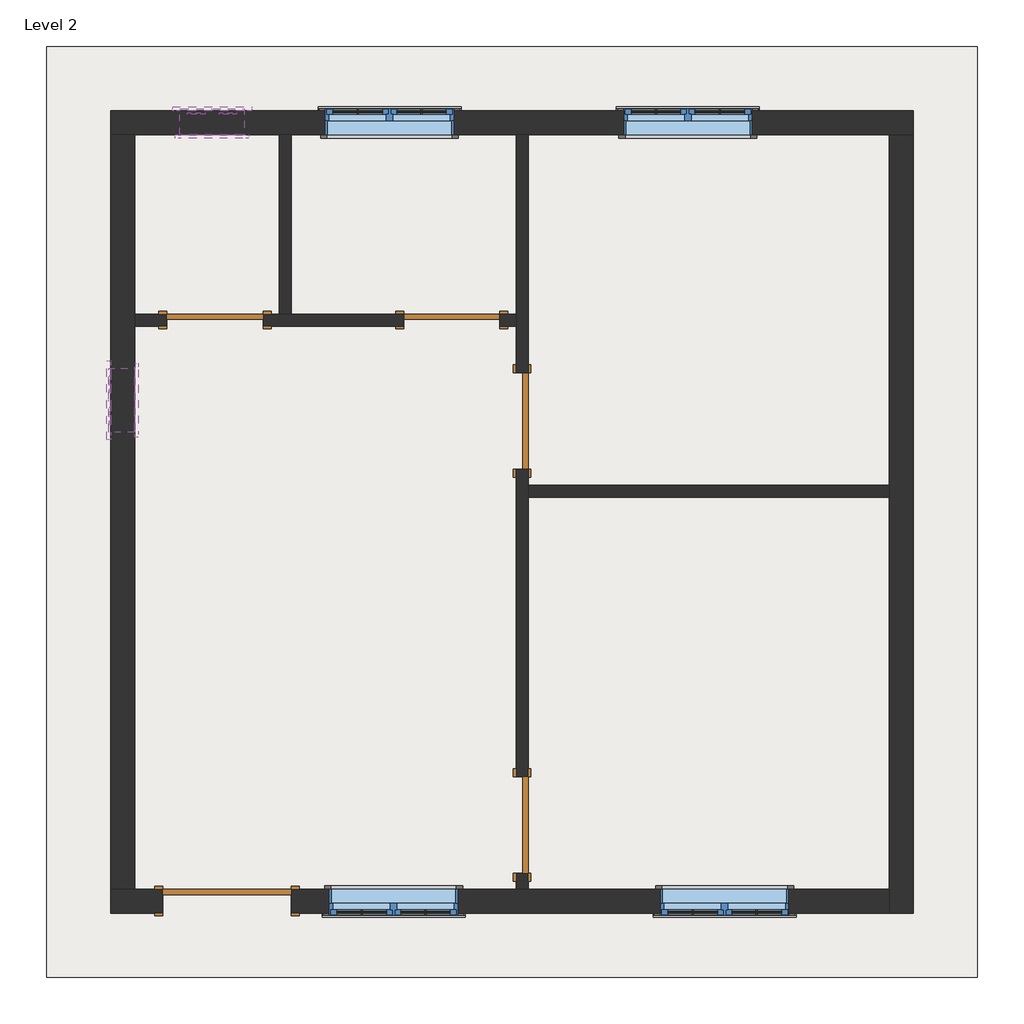
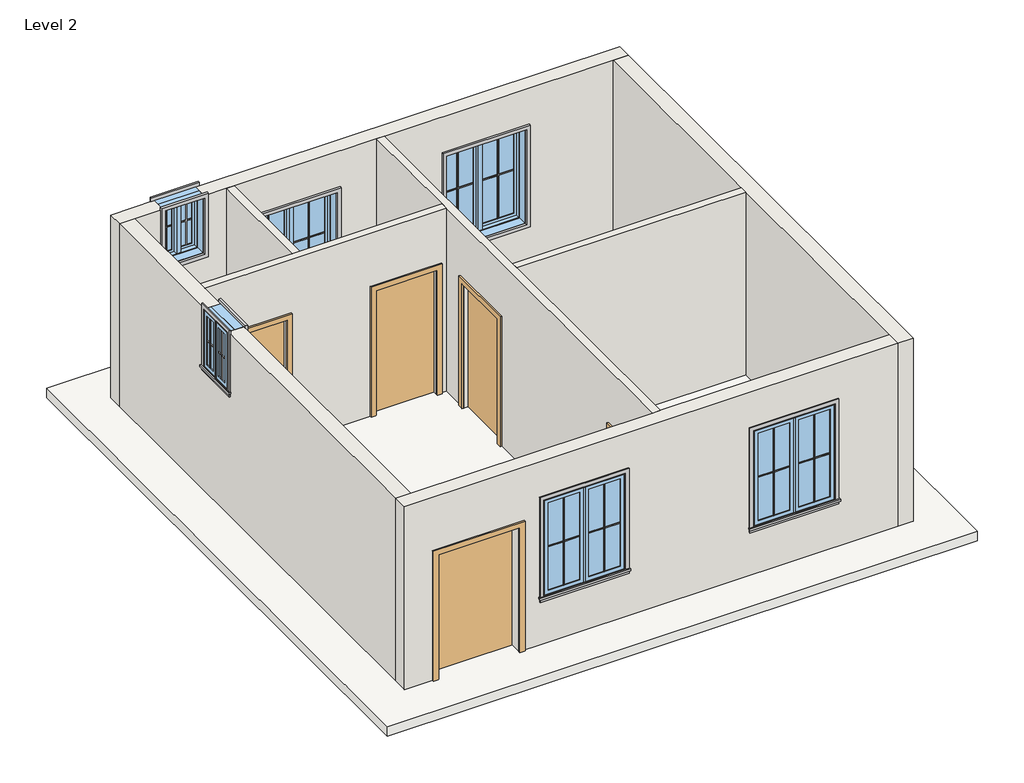
# One storey, incomplete: 24 proxies, 8 walls, 6 windows, 5 doors, 1 roof.
"""IFC4 building model written with IfcOpenShell, lengths in millimetres."""

from ifc_helpers import new_model, si_unit, frame, origin, place, context, project, spatial, polyline, outline, extrude, faceted_brep, transform, mapped, element, save
from components import muntin_pattern_2x2_muntin_pattern_2x2_6dad3731, muntin_pattern_2x2_muntin_pattern_2x2_a30a3345, muntin_pattern_2x2_muntin_pattern_2x2_53152e2c, muntin_pattern_2x2_muntin_pattern_2x2_e8f3e573, trim_window_exterior_flat_with_sill_92b9b949, trim_window_exterior_flat_with_sill_a665a915, trim_window_interior_flat_picture_frame_3bb882cf, trim_window_interior_flat_picture_frame_d485c387, door_e5f9f3c4, door_f4c4cdf2, window_c417fced, window_8377141f

model = new_model("IFC4")

# Units and contexts
model_context = context("Model", 3, world=origin())
ifc_project = project(units=[si_unit("LENGTHUNIT", "METRE", prefix="MILLI")], contexts=[model_context])

# Site, building, storey
site = spatial("IfcSite", under=ifc_project)
building = spatial("IfcBuilding", under=site)
storey = spatial("IfcBuildingStorey", under=building, Name="Level 2", Elevation=3048.0)

# Proxies
placement = place(None, origin())
muntin_pattern_2x2_muntin_pattern_2x2_shape = muntin_pattern_2x2_muntin_pattern_2x2_6dad3731(model_context)
element("IfcBuildingElementProxy", 1, Name="Muntin Pattern_2x2 : Muntin Pattern_2x2", ObjectType="Muntin Pattern_2x2 : Muntin Pattern_2x2", at=placement, inside=storey, context=model_context, shape_type="MappedRepresentation", body=[
    mapped(muntin_pattern_2x2_muntin_pattern_2x2_shape, transform((6192.8375, 13960.475, 4032.25), x_axis=(1.0, 0.0, 0.0), y_axis=(0.0, 1.0, 0.0), z_axis=(0.0, 0.0, 1.0))),
])
element("IfcBuildingElementProxy", 2, Name="Muntin Pattern_2x2 : Muntin Pattern_2x2", ObjectType="Muntin Pattern_2x2 : Muntin Pattern_2x2", at=placement, inside=storey, context=model_context, shape_type="MappedRepresentation", body=[
    mapped(muntin_pattern_2x2_muntin_pattern_2x2_shape, transform((7148.5125, 6359.525, 4032.25), x_axis=(-1.0, 0.0, 0.0), y_axis=(0.0, -1.0, 0.0), z_axis=(0.0, 0.0, 1.0))),
])
element("IfcBuildingElementProxy", 3, Name="Muntin Pattern_2x2 : Muntin Pattern_2x2", ObjectType="Muntin Pattern_2x2 : Muntin Pattern_2x2", at=placement, inside=storey, context=model_context, shape_type="MappedRepresentation", body=[
    mapped(muntin_pattern_2x2_muntin_pattern_2x2_shape, transform((4005.2625, 6359.525, 4032.25), x_axis=(-1.0, 0.0, 0.0), y_axis=(0.0, -1.0, 0.0), z_axis=(0.0, 0.0, 1.0))),
])
element("IfcBuildingElementProxy", 4, Name="Muntin Pattern_2x2 : Muntin Pattern_2x2", ObjectType="Muntin Pattern_2x2 : Muntin Pattern_2x2", at=placement, inside=storey, context=model_context, shape_type="MappedRepresentation", body=[
    mapped(muntin_pattern_2x2_muntin_pattern_2x2_shape, transform((3360.7375, 13960.475, 4032.25), x_axis=(1.0, 0.0, 0.0), y_axis=(0.0, 1.0, 0.0), z_axis=(0.0, 0.0, 1.0))),
])
muntin_pattern_2x2_muntin_pattern_2x2_2_shape = muntin_pattern_2x2_muntin_pattern_2x2_a30a3345(model_context)
element("IfcBuildingElementProxy", 5, Name="Muntin Pattern_2x2 : Muntin Pattern_2x2", ObjectType="Muntin Pattern_2x2 : Muntin Pattern_2x2", at=placement, inside=storey, context=model_context, shape_type="MappedRepresentation", body=[
    mapped(muntin_pattern_2x2_muntin_pattern_2x2_2_shape, transform((6799.2625, 13960.475, 4032.25), x_axis=(-1.0, 0.0, 0.0), y_axis=(0.0, -1.0, 0.0), z_axis=(0.0, 0.0, 1.0))),
])
element("IfcBuildingElementProxy", 6, Name="Muntin Pattern_2x2 : Muntin Pattern_2x2", ObjectType="Muntin Pattern_2x2 : Muntin Pattern_2x2", at=placement, inside=storey, context=model_context, shape_type="MappedRepresentation", body=[
    mapped(muntin_pattern_2x2_muntin_pattern_2x2_2_shape, transform((6542.0875, 6359.525, 4032.25), x_axis=(1.0, 0.0, 0.0), y_axis=(0.0, 1.0, 0.0), z_axis=(0.0, 0.0, 1.0))),
])
element("IfcBuildingElementProxy", 7, Name="Muntin Pattern_2x2 : Muntin Pattern_2x2", ObjectType="Muntin Pattern_2x2 : Muntin Pattern_2x2", at=placement, inside=storey, context=model_context, shape_type="MappedRepresentation", body=[
    mapped(muntin_pattern_2x2_muntin_pattern_2x2_2_shape, transform((3398.8375, 6359.525, 4032.25), x_axis=(1.0, 0.0, 0.0), y_axis=(0.0, 1.0, 0.0), z_axis=(0.0, 0.0, 1.0))),
])
element("IfcBuildingElementProxy", 8, Name="Muntin Pattern_2x2 : Muntin Pattern_2x2", ObjectType="Muntin Pattern_2x2 : Muntin Pattern_2x2", at=placement, inside=storey, context=model_context, shape_type="MappedRepresentation", body=[
    mapped(muntin_pattern_2x2_muntin_pattern_2x2_2_shape, transform((3967.1625, 13960.475, 4032.25), x_axis=(-1.0, 0.0, 0.0), y_axis=(0.0, -1.0, 0.0), z_axis=(0.0, 0.0, 1.0))),
])
muntin_pattern_2x2_muntin_pattern_2x2_3_shape = muntin_pattern_2x2_muntin_pattern_2x2_53152e2c(model_context)
element("IfcBuildingElementProxy", 9, Name="Muntin Pattern_2x2 : Muntin Pattern_2x2", ObjectType="Muntin Pattern_2x2 : Muntin Pattern_2x2", at=placement, inside=storey, context=model_context, shape_type="MappedRepresentation", body=[
    mapped(muntin_pattern_2x2_muntin_pattern_2x2_3_shape, transform((1025.525, 11069.6375, 5251.45), x_axis=(0.0, 1.0, 0.0), y_axis=(-1.0, 0.0, 0.0), z_axis=(0.0, 0.0, 1.0))),
])
element("IfcBuildingElementProxy", 10, Name="Muntin Pattern_2x2 : Muntin Pattern_2x2", ObjectType="Muntin Pattern_2x2 : Muntin Pattern_2x2", at=placement, inside=storey, context=model_context, shape_type="MappedRepresentation", body=[
    mapped(muntin_pattern_2x2_muntin_pattern_2x2_3_shape, transform((1827.2125, 13960.475, 5251.45), x_axis=(1.0, 0.0, 0.0), y_axis=(0.0, 1.0, 0.0), z_axis=(0.0, 0.0, 1.0))),
])
muntin_pattern_2x2_muntin_pattern_2x2_4_shape = muntin_pattern_2x2_muntin_pattern_2x2_e8f3e573(model_context)
element("IfcBuildingElementProxy", 11, Name="Muntin Pattern_2x2 : Muntin Pattern_2x2", ObjectType="Muntin Pattern_2x2 : Muntin Pattern_2x2", at=placement, inside=storey, context=model_context, shape_type="MappedRepresentation", body=[
    mapped(muntin_pattern_2x2_muntin_pattern_2x2_4_shape, transform((1025.525, 11371.2625, 5251.45), x_axis=(0.0, -1.0, 0.0), y_axis=(1.0, 0.0, 0.0), z_axis=(0.0, 0.0, 1.0))),
])
element("IfcBuildingElementProxy", 12, Name="Muntin Pattern_2x2 : Muntin Pattern_2x2", ObjectType="Muntin Pattern_2x2 : Muntin Pattern_2x2", at=placement, inside=storey, context=model_context, shape_type="MappedRepresentation", body=[
    mapped(muntin_pattern_2x2_muntin_pattern_2x2_4_shape, transform((2128.8375, 13960.475, 5251.45), x_axis=(-1.0, 0.0, 0.0), y_axis=(0.0, -1.0, 0.0), z_axis=(0.0, 0.0, 1.0))),
])
trim_window_exterior_flat_with_sill_shape = trim_window_exterior_flat_with_sill_92b9b949(model_context)
element("IfcBuildingElementProxy", 13, Name="Trim-Window-Exterior-Flat : with Sill", ObjectType="Trim-Window-Exterior-Flat : with Sill", at=placement, inside=storey, context=model_context, shape_type="MappedRepresentation", body=[
    mapped(trim_window_exterior_flat_with_sill_shape, transform((6496.05, 13970.0, 5486.4), x_axis=(-1.0, 0.0, 0.0), y_axis=(0.0, 0.0, 1.0), z_axis=(0.0, 1.0, 0.0))),
])
element("IfcBuildingElementProxy", 14, Name="Trim-Window-Exterior-Flat : with Sill", ObjectType="Trim-Window-Exterior-Flat : with Sill", at=placement, inside=storey, context=model_context, shape_type="MappedRepresentation", body=[
    mapped(trim_window_exterior_flat_with_sill_shape, transform((6845.3, 6350.0, 5486.4), x_axis=(1.0, 0.0, 0.0), y_axis=(0.0, 0.0, 1.0), z_axis=(0.0, -1.0, 0.0))),
])
element("IfcBuildingElementProxy", 15, Name="Trim-Window-Exterior-Flat : with Sill", ObjectType="Trim-Window-Exterior-Flat : with Sill", at=placement, inside=storey, context=model_context, shape_type="MappedRepresentation", body=[
    mapped(trim_window_exterior_flat_with_sill_shape, transform((3702.05, 6350.0, 5486.4), x_axis=(1.0, 0.0, 0.0), y_axis=(0.0, 0.0, 1.0), z_axis=(0.0, -1.0, 0.0))),
])
element("IfcBuildingElementProxy", 16, Name="Trim-Window-Exterior-Flat : with Sill", ObjectType="Trim-Window-Exterior-Flat : with Sill", at=placement, inside=storey, context=model_context, shape_type="MappedRepresentation", body=[
    mapped(trim_window_exterior_flat_with_sill_shape, transform((3663.95, 13970.0, 5486.4), x_axis=(-1.0, 0.0, 0.0), y_axis=(0.0, 0.0, 1.0), z_axis=(0.0, 1.0, 0.0))),
])
trim_window_exterior_flat_with_sill_2_shape = trim_window_exterior_flat_with_sill_a665a915(model_context)
element("IfcBuildingElementProxy", 17, Name="Trim-Window-Exterior-Flat : with Sill", ObjectType="Trim-Window-Exterior-Flat : with Sill", at=placement, inside=storey, context=model_context, shape_type="MappedRepresentation", body=[
    mapped(trim_window_exterior_flat_with_sill_2_shape, transform((1016.0, 11220.45, 6096.0), x_axis=(0.0, -1.0, 0.0), y_axis=(0.0, 0.0, 1.0), z_axis=(-1.0, 0.0, 0.0))),
])
element("IfcBuildingElementProxy", 18, Name="Trim-Window-Exterior-Flat : with Sill", ObjectType="Trim-Window-Exterior-Flat : with Sill", at=placement, inside=storey, context=model_context, shape_type="MappedRepresentation", body=[
    mapped(trim_window_exterior_flat_with_sill_2_shape, transform((1978.025, 13970.0, 6096.0), x_axis=(-1.0, 0.0, 0.0), y_axis=(0.0, 0.0, 1.0), z_axis=(0.0, 1.0, 0.0))),
])
trim_window_interior_flat_picture_frame_shape = trim_window_interior_flat_picture_frame_3bb882cf(model_context)
element("IfcBuildingElementProxy", 19, Name="Trim-Window-Interior-Flat : Picture Frame", ObjectType="Trim-Window-Interior-Flat : Picture Frame", at=placement, inside=storey, context=model_context, shape_type="MappedRepresentation", body=[
    mapped(trim_window_interior_flat_picture_frame_shape, transform((6496.05, 13741.4, 5486.4), x_axis=(1.0, 0.0, 0.0), y_axis=(0.0, 0.0, 1.0), z_axis=(0.0, -1.0, 0.0))),
])
element("IfcBuildingElementProxy", 20, Name="Trim-Window-Interior-Flat : Picture Frame", ObjectType="Trim-Window-Interior-Flat : Picture Frame", at=placement, inside=storey, context=model_context, shape_type="MappedRepresentation", body=[
    mapped(trim_window_interior_flat_picture_frame_shape, transform((6845.3, 6578.6, 5486.4), x_axis=(-1.0, 0.0, 0.0), y_axis=(0.0, 0.0, 1.0), z_axis=(0.0, 1.0, 0.0))),
])
element("IfcBuildingElementProxy", 21, Name="Trim-Window-Interior-Flat : Picture Frame", ObjectType="Trim-Window-Interior-Flat : Picture Frame", at=placement, inside=storey, context=model_context, shape_type="MappedRepresentation", body=[
    mapped(trim_window_interior_flat_picture_frame_shape, transform((3702.05, 6578.6, 5486.4), x_axis=(-1.0, 0.0, 0.0), y_axis=(0.0, 0.0, 1.0), z_axis=(0.0, 1.0, 0.0))),
])
element("IfcBuildingElementProxy", 22, Name="Trim-Window-Interior-Flat : Picture Frame", ObjectType="Trim-Window-Interior-Flat : Picture Frame", at=placement, inside=storey, context=model_context, shape_type="MappedRepresentation", body=[
    mapped(trim_window_interior_flat_picture_frame_shape, transform((3663.95, 13741.4, 5486.4), x_axis=(1.0, 0.0, 0.0), y_axis=(0.0, 0.0, 1.0), z_axis=(0.0, -1.0, 0.0))),
])
trim_window_interior_flat_picture_frame_2_shape = trim_window_interior_flat_picture_frame_d485c387(model_context)
element("IfcBuildingElementProxy", 23, Name="Trim-Window-Interior-Flat : Picture Frame", ObjectType="Trim-Window-Interior-Flat : Picture Frame", at=placement, inside=storey, context=model_context, shape_type="MappedRepresentation", body=[
    mapped(trim_window_interior_flat_picture_frame_2_shape, transform((1244.6, 11220.45, 6096.0), x_axis=(0.0, 1.0, 0.0), y_axis=(0.0, 0.0, 1.0), z_axis=(1.0, 0.0, 0.0))),
])
element("IfcBuildingElementProxy", 24, Name="Trim-Window-Interior-Flat : Picture Frame", ObjectType="Trim-Window-Interior-Flat : Picture Frame", at=placement, inside=storey, context=model_context, shape_type="MappedRepresentation", body=[
    mapped(trim_window_interior_flat_picture_frame_2_shape, transform((1978.025, 13741.4, 6096.0), x_axis=(1.0, 0.0, 0.0), y_axis=(0.0, 0.0, 1.0), z_axis=(0.0, -1.0, 0.0))),
])

# Doors
door_shape = door_e5f9f3c4(model_context)
element("IfcDoor", 25, ObjectType="Single-Flush : 36\" x 84\"", at=placement, inside=storey, context=model_context, shape_type="MappedRepresentation", body=[
    mapped(door_shape, transform((2006.6, 11982.45, 3048.0), x_axis=(1.0, 0.0, 0.0), y_axis=(0.0, 1.0, 0.0), z_axis=(0.0, 0.0, 1.0))),
])
element("IfcDoor", 26, ObjectType="Single-Flush : 36\" x 84\"", at=placement, inside=storey, context=model_context, shape_type="MappedRepresentation", body=[
    mapped(door_shape, transform((4254.5, 11982.45, 3048.0), x_axis=(1.0, 0.0, 0.0), y_axis=(0.0, 1.0, 0.0), z_axis=(0.0, 0.0, 1.0))),
])
element("IfcDoor", 27, ObjectType="Single-Flush : 36\" x 84\"", at=placement, inside=storey, context=model_context, shape_type="MappedRepresentation", body=[
    mapped(door_shape, transform((4921.25, 11023.6, 3048.0), x_axis=(0.0, -1.0, 0.0), y_axis=(1.0, 0.0, 0.0), z_axis=(0.0, 0.0, 1.0))),
])
element("IfcDoor", 28, ObjectType="Single-Flush : 36\" x 84\"", at=placement, inside=storey, context=model_context, shape_type="MappedRepresentation", body=[
    mapped(door_shape, transform((4921.25, 7188.2, 3048.0), x_axis=(0.0, -1.0, 0.0), y_axis=(1.0, 0.0, 0.0), z_axis=(0.0, 0.0, 1.0))),
])
door_2_shape = door_f4c4cdf2(model_context)
element("IfcDoor", 29, ObjectType="Single-Flush : 48\" x 84\"", at=placement, inside=storey, context=model_context, shape_type="MappedRepresentation", body=[
    mapped(door_2_shape, transform((2120.9, 6464.3, 3048.0), x_axis=(-1.0, 0.0, 0.0), y_axis=(0.0, -1.0, 0.0), z_axis=(0.0, 0.0, 1.0))),
])

# Roof
element("IfcRoof", 30, ObjectType="Generic - 12\"", at=placement, inside=storey, context=model_context, shape_type="SweptSolid", body=[
    extrude(outline(polyline([(406.4, 14579.6), (9245.6, 14579.6), (9245.6, 5740.4), (406.4, 5740.4), (406.4, 14579.6)])), frame((0.0, 0.0, 3048.0), z_axis=(0.0, 0.0, 1.0), x_axis=(1.0, 0.0, 0.0)), (0.0, 0.0, 1.0), 152.4),
])

# Walls
element("IfcWall", 31, ObjectType="Generic - 5\"", at=placement, inside=storey, context=model_context, shape_type="SweptSolid", body=[
    extrude(outline(polyline([(2616.2, 12039.6), (2616.2, 13741.4), (2730.5, 13741.4), (2730.5, 12039.6), (2616.2, 12039.6)])), frame((0.0, 0.0, 3048.0), z_axis=(0.0, 0.0, 1.0), x_axis=(1.0, 0.0, 0.0)), (0.0, 0.0, 1.0), 3048.0),
])
element("IfcWall", 32, ObjectType="Generic - 5\"", at=placement, inside=storey, context=model_context, shape_type="Brep", body=[
    faceted_brep([(4711.7, 11925.3, 5181.6), (4711.7, 11925.3, 3048.0), (4864.1, 11925.3, 3048.0), (4864.1, 11925.3, 6096.0), (1244.6, 11925.3, 6096.0), (1244.6, 11925.3, 3048.0), (1549.4, 11925.3, 3048.0), (1549.4, 11925.3, 5181.6), (2463.8, 11925.3, 5181.6), (2463.8, 11925.3, 3048.0), (3797.3, 11925.3, 3048.0), (3797.3, 11925.3, 5181.6), (4864.1, 12039.6, 3048.0), (4711.7, 12039.6, 3048.0), (4711.7, 12039.6, 5181.6), (3797.3, 12039.6, 5181.6), (3797.3, 12039.6, 3048.0), (2730.5, 12039.6, 3048.0), (2616.2, 12039.6, 3048.0), (2463.8, 12039.6, 3048.0), (2463.8, 12039.6, 5181.6), (1549.4, 12039.6, 5181.6), (1549.4, 12039.6, 3048.0), (1244.6, 12039.6, 3048.0), (1244.6, 12039.6, 6096.0), (2616.2, 12039.6, 6096.0), (2730.5, 12039.6, 6096.0), (4864.1, 12039.6, 6096.0)], [[[0, 1, 2, 3, 4, 5, 6, 7, 8, 9, 10, 11]], [[12, 13, 14, 15, 16, 17, 18, 19, 20, 21, 22, 23, 24, 25, 26, 27]], [[6, 5, 23, 22]], [[10, 9, 19, 18, 17, 16]], [[2, 1, 13, 12]], [[4, 3, 27, 26, 25, 24]], [[5, 4, 24, 23]], [[3, 2, 12, 27]], [[20, 19, 9, 8]], [[21, 20, 8, 7]], [[22, 21, 7, 6]], [[14, 13, 1, 0]], [[15, 14, 0, 11]], [[16, 15, 11, 10]]]),
])
element("IfcWall", 33, ObjectType="Generic - 5\"", at=placement, inside=storey, context=model_context, shape_type="Brep", body=[
    faceted_brep([(4864.1, 6731.0, 5181.6), (4864.1, 6731.0, 3048.0), (4864.1, 6578.6, 3048.0), (4864.1, 6578.6, 6096.0), (4864.1, 11925.3, 6096.0), (4864.1, 12039.6, 6096.0), (4864.1, 13741.4, 6096.0), (4864.1, 13741.4, 3048.0), (4864.1, 12039.6, 3048.0), (4864.1, 11925.3, 3048.0), (4864.1, 11480.8, 3048.0), (4864.1, 11480.8, 5181.6), (4864.1, 10566.4, 5181.6), (4864.1, 10566.4, 3048.0), (4864.1, 7645.4, 3048.0), (4864.1, 7645.4, 5181.6), (4978.4, 6578.6, 3048.0), (4978.4, 6731.0, 3048.0), (4978.4, 6731.0, 5181.6), (4978.4, 7645.4, 5181.6), (4978.4, 7645.4, 3048.0), (4978.4, 10299.7, 3048.0), (4978.4, 10414.0, 3048.0), (4978.4, 10566.4, 3048.0), (4978.4, 10566.4, 5181.6), (4978.4, 11480.8, 5181.6), (4978.4, 11480.8, 3048.0), (4978.4, 13741.4, 3048.0), (4978.4, 13741.4, 6096.0), (4978.4, 10414.0, 6096.0), (4978.4, 10299.7, 6096.0), (4978.4, 6578.6, 6096.0)], [[[0, 1, 2, 3, 4, 5, 6, 7, 8, 9, 10, 11, 12, 13, 14, 15]], [[16, 17, 18, 19, 20, 21, 22, 23, 24, 25, 26, 27, 28, 29, 30, 31]], [[10, 9, 8, 7, 27, 26]], [[14, 13, 23, 22, 21, 20]], [[2, 1, 17, 16]], [[6, 5, 4, 3, 31, 30, 29, 28]], [[7, 6, 28, 27]], [[3, 2, 16, 31]], [[24, 23, 13, 12]], [[25, 24, 12, 11]], [[26, 25, 11, 10]], [[18, 17, 1, 0]], [[19, 18, 0, 15]], [[20, 19, 15, 14]]]),
])
element("IfcWall", 34, ObjectType="Generic - 5\"", at=placement, inside=storey, context=model_context, shape_type="SweptSolid", body=[
    extrude(outline(polyline([(8407.4, 10299.7), (4978.4, 10299.7), (4978.4, 10414.0), (8407.4, 10414.0), (8407.4, 10299.7)])), frame((0.0, 0.0, 3048.0), z_axis=(0.0, 0.0, 1.0), x_axis=(1.0, 0.0, 0.0)), (0.0, 0.0, 1.0), 3048.0),
])
element("IfcWall", 35, ObjectType="Generic - 8\"", at=placement, inside=storey, context=model_context, shape_type="Brep", body=[
    faceted_brep([(1016.0, 13741.4, 3048.0), (1244.6, 13741.4, 3048.0), (2616.2, 13741.4, 3048.0), (2730.5, 13741.4, 3048.0), (4864.1, 13741.4, 3048.0), (4978.4, 13741.4, 3048.0), (8407.4, 13741.4, 3048.0), (8636.0, 13741.4, 3048.0), (8636.0, 13741.4, 6096.0), (8407.4, 13741.4, 6096.0), (4978.4, 13741.4, 6096.0), (4864.1, 13741.4, 6096.0), (2730.5, 13741.4, 6096.0), (2616.2, 13741.4, 6096.0), (2282.825, 13741.4, 6096.0), (2282.825, 13741.4, 5181.6), (1673.225, 13741.4, 5181.6), (1673.225, 13741.4, 6096.0), (1244.6, 13741.4, 6096.0), (1016.0, 13741.4, 6096.0), (7105.65, 13741.4, 5486.4), (7105.65, 13741.4, 3962.4), (5886.45, 13741.4, 3962.4), (5886.45, 13741.4, 5486.4), (4273.55, 13741.4, 5486.4), (4273.55, 13741.4, 3962.4), (3054.35, 13741.4, 3962.4), (3054.35, 13741.4, 5486.4), (8636.0, 13970.0, 3048.0), (1016.0, 13970.0, 3048.0), (1016.0, 13970.0, 6096.0), (1673.225, 13970.0, 6096.0), (1673.225, 13970.0, 5181.6), (2282.825, 13970.0, 5181.6), (2282.825, 13970.0, 6096.0), (8636.0, 13970.0, 6096.0), (7105.65, 13970.0, 3962.4), (7105.65, 13970.0, 5486.4), (5886.45, 13970.0, 5486.4), (5886.45, 13970.0, 3962.4), (4273.55, 13970.0, 3962.4), (4273.55, 13970.0, 5486.4), (3054.35, 13970.0, 5486.4), (3054.35, 13970.0, 3962.4)], [[[0, 1, 2, 3, 4, 5, 6, 7, 8, 9, 10, 11, 12, 13, 14, 15, 16, 17, 18, 19], [20, 21, 22, 23], [24, 25, 26, 27]], [[28, 29, 30, 31, 32, 33, 34, 35], [36, 37, 38, 39], [40, 41, 42, 43]], [[7, 6, 5, 4, 3, 2, 1, 0, 29, 28]], [[8, 35, 34, 14, 13, 12, 11, 10, 9]], [[30, 19, 18, 17, 31]], [[8, 7, 28, 35]], [[0, 19, 30, 29]], [[21, 20, 37, 36]], [[22, 21, 36, 39]], [[23, 22, 39, 38]], [[20, 23, 38, 37]], [[25, 24, 41, 40]], [[26, 25, 40, 43]], [[27, 26, 43, 42]], [[24, 27, 42, 41]], [[33, 15, 14, 34]], [[15, 33, 32, 16]], [[16, 32, 31, 17]]]),
])
element("IfcWall", 36, ObjectType="Generic - 8\"", at=placement, inside=storey, context=model_context, shape_type="Brep", body=[
    faceted_brep([(8407.4, 13741.4, 3048.0), (8407.4, 10414.0, 3048.0), (8407.4, 10299.7, 3048.0), (8407.4, 6578.6, 3048.0), (8407.4, 6350.0, 3048.0), (8407.4, 6350.0, 6096.0), (8407.4, 6578.6, 6096.0), (8407.4, 10299.7, 6096.0), (8407.4, 10414.0, 6096.0), (8407.4, 13741.4, 6096.0), (8636.0, 13741.4, 3048.0), (8636.0, 13741.4, 6096.0), (8636.0, 6350.0, 6096.0), (8636.0, 6350.0, 3048.0)], [[[0, 1, 2, 3, 4, 5, 6, 7, 8, 9]], [[10, 11, 12, 13]], [[4, 3, 2, 1, 0, 10, 13]], [[9, 8, 7, 6, 5, 12, 11]], [[0, 9, 11, 10]], [[5, 4, 13, 12]]]),
])
element("IfcWall", 37, ObjectType="Generic - 8\"", at=placement, inside=storey, context=model_context, shape_type="Brep", body=[
    faceted_brep([(1511.3, 6578.6, 5181.6), (1511.3, 6578.6, 3048.0), (1244.6, 6578.6, 3048.0), (1016.0, 6578.6, 3048.0), (1016.0, 6578.6, 6096.0), (1244.6, 6578.6, 6096.0), (4864.1, 6578.6, 6096.0), (4978.4, 6578.6, 6096.0), (8407.4, 6578.6, 6096.0), (8407.4, 6578.6, 3048.0), (4978.4, 6578.6, 3048.0), (4864.1, 6578.6, 3048.0), (2730.5, 6578.6, 3048.0), (2730.5, 6578.6, 5181.6), (6235.7, 6578.6, 5486.4), (6235.7, 6578.6, 3962.4), (7454.9, 6578.6, 3962.4), (7454.9, 6578.6, 5486.4), (3092.45, 6578.6, 5486.4), (3092.45, 6578.6, 3962.4), (4311.65, 6578.6, 3962.4), (4311.65, 6578.6, 5486.4), (1016.0, 6350.0, 3048.0), (1511.3, 6350.0, 3048.0), (1511.3, 6350.0, 5181.6), (2730.5, 6350.0, 5181.6), (2730.5, 6350.0, 3048.0), (8407.4, 6350.0, 3048.0), (8407.4, 6350.0, 6096.0), (1016.0, 6350.0, 6096.0), (6235.7, 6350.0, 5486.4), (7454.9, 6350.0, 5486.4), (7454.9, 6350.0, 3962.4), (6235.7, 6350.0, 3962.4), (3092.45, 6350.0, 5486.4), (4311.65, 6350.0, 5486.4), (4311.65, 6350.0, 3962.4), (3092.45, 6350.0, 3962.4)], [[[0, 1, 2, 3, 4, 5, 6, 7, 8, 9, 10, 11, 12, 13], [14, 15, 16, 17], [18, 19, 20, 21]], [[22, 23, 24, 25, 26, 27, 28, 29], [30, 31, 32, 33], [34, 35, 36, 37]], [[3, 2, 1, 23, 22]], [[12, 11, 10, 9, 27, 26]], [[8, 7, 6, 5, 4, 29, 28]], [[9, 8, 28, 27]], [[4, 3, 22, 29]], [[24, 23, 1, 0]], [[25, 24, 0, 13]], [[26, 25, 13, 12]], [[15, 14, 30, 33]], [[16, 15, 33, 32]], [[17, 16, 32, 31]], [[14, 17, 31, 30]], [[19, 18, 34, 37]], [[20, 19, 37, 36]], [[21, 20, 36, 35]], [[18, 21, 35, 34]]]),
])
element("IfcWall", 38, ObjectType="Generic - 8\"", at=placement, inside=storey, context=model_context, shape_type="Brep", body=[
    faceted_brep([(1244.6, 6578.6, 3048.0), (1244.6, 11925.3, 3048.0), (1244.6, 12039.6, 3048.0), (1244.6, 13741.4, 3048.0), (1244.6, 13741.4, 6096.0), (1244.6, 12039.6, 6096.0), (1244.6, 11925.3, 6096.0), (1244.6, 11525.25, 6096.0), (1244.6, 11525.25, 5181.6), (1244.6, 10915.65, 5181.6), (1244.6, 10915.65, 6096.0), (1244.6, 6578.6, 6096.0), (1016.0, 13741.4, 3048.0), (1016.0, 6578.6, 3048.0), (1016.0, 6578.6, 6096.0), (1016.0, 10915.65, 6096.0), (1016.0, 10915.65, 5181.6), (1016.0, 11525.25, 5181.6), (1016.0, 11525.25, 6096.0), (1016.0, 13741.4, 6096.0)], [[[0, 1, 2, 3, 4, 5, 6, 7, 8, 9, 10, 11]], [[12, 13, 14, 15, 16, 17, 18, 19]], [[3, 2, 1, 0, 13, 12]], [[14, 11, 10, 15]], [[4, 19, 18, 7, 6, 5]], [[4, 3, 12, 19]], [[0, 11, 14, 13]], [[17, 8, 7, 18]], [[8, 17, 16, 9]], [[9, 16, 15, 10]]]),
])

# Windows
window_shape = window_c417fced(model_context)
element("IfcWindow", 39, ObjectType="Window-Casement-Double : 24\" x 36\"", at=placement, inside=storey, context=model_context, shape_type="MappedRepresentation", body=[
    mapped(window_shape, transform((1130.3, 11220.45, 4267.2), x_axis=(0.0, 1.0, 0.0), y_axis=(-1.0, 0.0, 0.0), z_axis=(0.0, 0.0, 1.0))),
])
element("IfcWindow", 40, ObjectType="Window-Casement-Double : 24\" x 36\"", at=placement, inside=storey, context=model_context, shape_type="MappedRepresentation", body=[
    mapped(window_shape, transform((1978.025, 13855.7, 4267.2), x_axis=(1.0, 0.0, 0.0), y_axis=(0.0, 1.0, 0.0), z_axis=(0.0, 0.0, 1.0))),
])
window_2_shape = window_8377141f(model_context)
element("IfcWindow", 41, ObjectType="Window-Casement-Double : 48\" x 60\"", at=placement, inside=storey, context=model_context, shape_type="MappedRepresentation", body=[
    mapped(window_2_shape, transform((6496.05, 13855.7, 3048.0), x_axis=(1.0, 0.0, 0.0), y_axis=(0.0, 1.0, 0.0), z_axis=(0.0, 0.0, 1.0))),
])
element("IfcWindow", 42, ObjectType="Window-Casement-Double : 48\" x 60\"", at=placement, inside=storey, context=model_context, shape_type="MappedRepresentation", body=[
    mapped(window_2_shape, transform((6845.3, 6464.3, 3048.0), x_axis=(-1.0, 0.0, 0.0), y_axis=(0.0, -1.0, 0.0), z_axis=(0.0, 0.0, 1.0))),
])
element("IfcWindow", 43, ObjectType="Window-Casement-Double : 48\" x 60\"", at=placement, inside=storey, context=model_context, shape_type="MappedRepresentation", body=[
    mapped(window_2_shape, transform((3702.05, 6464.3, 3048.0), x_axis=(-1.0, 0.0, 0.0), y_axis=(0.0, -1.0, 0.0), z_axis=(0.0, 0.0, 1.0))),
])
element("IfcWindow", 44, ObjectType="Window-Casement-Double : 48\" x 60\"", at=placement, inside=storey, context=model_context, shape_type="MappedRepresentation", body=[
    mapped(window_2_shape, transform((3663.95, 13855.7, 3048.0), x_axis=(1.0, 0.0, 0.0), y_axis=(0.0, 1.0, 0.0), z_axis=(0.0, 0.0, 1.0))),
])

save(model, "model.ifc")

# Revit data of these elements
# Type "Muntin Pattern_2x2 : Muntin Pattern_2x2"
#   Width [instance default] = 4' - 0"
#   Thickness = 0' - 0 1/2"
#   Height [instance default] = 4' - 0"
#   Distance = 0' - 0 3/4"
#   Interior Material [instance default] = none
#   Exterior Material [instance default] = none
#   Default Elevation = 0
# Type "Trim-Window-Exterior-Flat : with Sill"
#   Trim Width = 0' - 2 1/4"
#   Trim Thickness_Picture Frame = 0' - 1 1/4"
#   Trim Thickness_with Sill = 0' - 0 3/4"
#   Sill Thickness = 0' - 1 1/4"
#   Opening Width [instance default] = 2' - 0"
#   Opening Height [instance default] = 3' - 0"
#   Default Elevation = 4' - 0"
#   Sill = yes
#   Picture Frame = no
#   Trim Material [instance default] = none
# Type "Trim-Window-Interior-Flat : Picture Frame"
#   Trim Thickness_Picture Frame = 0' - 1 1/4"
#   Trim Width = 0' - 2 1/4"
#   Trim Thickness_with Sill = 0' - 0 3/4"
#   Sill Thickness = 0' - 1 1/4"
#   Opening Width [instance default] = 2' - 0"
#   Opening Height [instance default] = 3' - 0"
#   Default Elevation = 4' - 0"
#   Sill = no
#   Picture Frame = yes
#   Trim Material [instance default] = none
# Type "Single-Flush : 36\" x 84\""
#   Type Mark = "1"
#   Construction Type Id = "MDOOR"
#   Assembly Code = "C1020"
#   Analytic Construction = "Metal"
#   Thickness = 0' - 2"
#   Heat Transfer Coefficient (U) = 0.651978 BTU/(h·ft²·°F)
#   Height = 7' - 0"
#   Trim Projection Ext = 0' - 1"
#   Trim Projection Int = 0' - 1"
#   Trim Width = 0' - 3"
#   Width = 3' - 0"
#   Define Thermal Properties by = 1
#   Define Thermal Properties by = 1
#   Door Material = Door - Panel
#   Frame Material = Door - Frame
#   Visual Light Transmittance = 0
#   Solar Heat Gain Coefficient = 0
#   Function = (empty or 0)
#   Wall Closure = (empty or 0)
# Type "Single-Flush : 48\" x 84\""
#   Type Mark = "5"
#   Construction Type Id = "MDOOR"
#   Assembly Code = "C1020"
#   Analytic Construction = "Metal"
#   Thickness = 0' - 2"
#   Heat Transfer Coefficient (U) = 0.651978 BTU/(h·ft²·°F)
#   Height = 7' - 0"
#   Trim Projection Ext = 0' - 1"
#   Trim Projection Int = 0' - 1"
#   Trim Width = 0' - 3"
#   Width = 4' - 0"
#   Define Thermal Properties by = 1
#   Define Thermal Properties by = 1
#   Door Material = Door - Panel
#   Frame Material = Door - Frame
#   Visual Light Transmittance = 0
#   Solar Heat Gain Coefficient = 0
#   Function = (empty or 0)
#   Wall Closure = (empty or 0)
# Type "Generic - 12\""
#   Assembly Code = "B1020"
#   Layers, outside or top first: 0' - 6" no material (function 1)
# Type "Generic - 5\""
#   Assembly Code = "B2010"
#   Layers, outside or top first: 0' - 4 1/2" no material (function 1)
# Type "Generic - 8\""
#   Assembly Code = "B2010"
#   Layers, outside or top first: 0' - 9" "Parking Stripe" (function 1)
# Type "Window-Casement-Double : 24\" x 36\""
#   Type Mark = "14"
#   Fire Rating = "0.5h"
#   Assembly Code = "B2020100"
#   Analytic Construction = "Double glazing - domestic"
#   Frame Extension [instance default] = 0' - 0 1/4"
#   Window Inset [instance default] = 0' - 0"
#   Wall Thickness [instance default] = 0' - 6"
#   Interior Wall Closure [instance default] = 0' - 2 1/4"
#   Half Width = 1' - 0"
#   Visual Light Transmittance = 0.81
#   Thermal Resistance (R) = 1.8146 (h·ft²·°F)/BTU
#   Solar Heat Gain Coefficient = 0.76
#   Rough Width = 2' - 0 1/2"
#   Rough Height = 3' - 0 1/2"
#   Height = 3' - 0"
#   Heat Transfer Coefficient (U) = 0.5511 BTU/(h·ft²·°F)
#   Exterior Wall Closure [instance default] = 0' - 1 1/4"
#   Extension Jamb [instance default] = 0' - 2 1/4"
#   Default Sill Height = 3' - 0"
#   Width = 2' - 0"
#   Define Thermal Properties by = 0
#   Muntin Visibility = yes
#   Interior Trim Visibility [instance default] = yes
#   Exterior Trim Visibility [instance default] = yes
#   Extension Jamb Visibility [instance default] = yes
#   Interior Trim Material = Wood - Stained
#   Muntin Pattern = Muntin Pattern_2x2 : Muntin Pattern_2x2
#   Interior Trim = Trim-Window-Interior-Flat : Picture Frame
#   Interior Frame Material = Wood - Stained
#   Glass Panel Material = Glass
#   Exterior Trim Material = Clad - White
#   Exterior Trim = Trim-Window-Exterior-Flat : with Sill
#   Exterior Frame Material = Clad - White
#   Wall Closure = (empty or 0)
# Type "Window-Casement-Double : 48\" x 60\""
#   Type Mark = "17"
#   Fire Rating = "0.5h"
#   Assembly Code = "B2020100"
#   Analytic Construction = "Double glazing - domestic"
#   Frame Extension [instance default] = 0' - 0 1/4"
#   Window Inset [instance default] = 0' - 0"
#   Wall Thickness [instance default] = 0' - 6"
#   Interior Wall Closure [instance default] = 0' - 2 1/4"
#   Half Width = 2' - 0"
#   Visual Light Transmittance = 0.81
#   Thermal Resistance (R) = 1.8146 (h·ft²·°F)/BTU
#   Solar Heat Gain Coefficient = 0.76
#   Rough Width = 4' - 0 1/2"
#   Rough Height = 5' - 0 1/2"
#   Height = 5' - 0"
#   Heat Transfer Coefficient (U) = 0.5511 BTU/(h·ft²·°F)
#   Exterior Wall Closure [instance default] = 0' - 1 1/4"
#   Extension Jamb [instance default] = 0' - 2 1/4"
#   Default Sill Height = 3' - 0"
#   Width = 4' - 0"
#   Define Thermal Properties by = 0
#   Muntin Visibility = yes
#   Interior Trim Visibility [instance default] = yes
#   Exterior Trim Visibility [instance default] = yes
#   Extension Jamb Visibility [instance default] = yes
#   Interior Trim Material = Wood - Stained
#   Muntin Pattern = Muntin Pattern_2x2 : Muntin Pattern_2x2
#   Interior Trim = Trim-Window-Interior-Flat : Picture Frame
#   Interior Frame Material = Wood - Stained
#   Glass Panel Material = Glass
#   Exterior Trim Material = Clad - White
#   Exterior Trim = Trim-Window-Exterior-Flat : with Sill
#   Exterior Frame Material = Clad - White
#   Wall Closure = (empty or 0)
# Elements 1, 2, 3, 4, 5, 6, 7, 8 (IfcBuildingElementProxy, "Muntin Pattern_2x2 : Muntin Pattern_2x2")
#   Width = 1' - 6 5/8"
#   Height = 4' - 6 1/2"
#   Interior Material = Wood - Stained
#   Exterior Material = Clad - White
#   Phase Created = New Construction
#   Materials on its faces: "Clad - White", "Wood - Stained"
# Elements 9, 10, 11, 12 (IfcBuildingElementProxy, "Muntin Pattern_2x2 : Muntin Pattern_2x2")
#   Width = 0' - 6 5/8"
#   Height = 2' - 6 1/2"
#   Interior Material = Wood - Stained
#   Exterior Material = Clad - White
#   Phase Created = New Construction
#   Materials on its faces: "Clad - White", "Wood - Stained"
# Elements 13, 14, 15, 16 (IfcBuildingElementProxy, "Trim-Window-Exterior-Flat : with Sill")
#   Opening Width = 4' - 0"
#   Opening Height = 5' - 0"
#   Trim Material = Clad - White
#   Phase Created = New Construction
#   Materials on its faces: "Clad - White"
# Elements 17, 18 (IfcBuildingElementProxy, "Trim-Window-Exterior-Flat : with Sill")
#   Opening Width = 2' - 0"
#   Opening Height = 3' - 0"
#   Trim Material = Clad - White
#   Phase Created = New Construction
#   Materials on its faces: "Clad - White"
# Elements 19, 20, 21, 22 (IfcBuildingElementProxy, "Trim-Window-Interior-Flat : Picture Frame")
#   Opening Width = 4' - 0"
#   Opening Height = 5' - 0"
#   Trim Material = Wood - Stained
#   Phase Created = New Construction
#   Materials on its faces: "Wood - Stained"
# Elements 23, 24 (IfcBuildingElementProxy, "Trim-Window-Interior-Flat : Picture Frame")
#   Opening Width = 2' - 0"
#   Opening Height = 3' - 0"
#   Trim Material = Wood - Stained
#   Phase Created = New Construction
#   Materials on its faces: "Wood - Stained"
# Elements 25, 26, 27, 28 (IfcDoor, "Single-Flush : 36\" x 84\"")
#   Phase Created = New Construction
#   Materials on its faces: "Door - Frame", "Door - Panel"
# Element 29 (IfcDoor, "Single-Flush : 48\" x 84\"")
#   Phase Created = New Construction
#   Materials on its faces: "Door - Frame", "Door - Panel"
# Element 30 (IfcRoof, "Generic - 12\"")
#   built-in parameter 1001705 = 10.5 (stored number, unit not read)
#   built-in parameter 1001710 = 33615
#   Phase Created = New Construction
#   Materials on its faces: "Textile - Linen, Smooth", "Wood Planks"
# Elements 31, 32, 33, 34 (IfcWall, "Generic - 5\"")
#   Top Offset = 0' - 0"
#   Base Offset = 0' - 0"
#   wall height = 10' - 0"
#   Phase Created = New Construction
#   Base Constraint = Level 2
#   Top Constraint = Level 3
#   Materials on its faces: "Default Wall"
# Elements 35, 36, 37, 38 (IfcWall, "Generic - 8\"")
#   Top Offset = 0' - 0"
#   Base Offset = 0' - 0"
#   Unconnected Height = 10' - 0"
#   wall height = 10' - 0"
#   Phase Created = New Construction
#   Base Constraint = Level 2
#   Materials on its faces: "Parking Stripe", "Wood Planks"
# Element 39 (IfcWindow, "Window-Casement-Double : 24\" x 36\"")
#   Mark = "11"
#   Window Inset = 0' - 0"
#   Interior Wall Closure = 0' - 2 1/4"
#   Frame Extension = 0' - 0 1/4"
#   Exterior Wall Closure = 0' - 1 1/4"
#   Interior Trim Visibility = yes
#   Exterior Trim Visibility = yes
#   Phase Created = New Construction
#   Materials on its faces: "Wood - Stained", "Glass", "Clad - White"
# Element 40 (IfcWindow, "Window-Casement-Double : 24\" x 36\"")
#   Mark = "12"
#   Window Inset = 0' - 0"
#   Interior Wall Closure = 0' - 2 1/4"
#   Frame Extension = 0' - 0 1/4"
#   Exterior Wall Closure = 0' - 1 1/4"
#   Interior Trim Visibility = yes
#   Exterior Trim Visibility = yes
#   Phase Created = New Construction
#   Materials on its faces: "Wood - Stained", "Glass", "Clad - White"
# Element 41 (IfcWindow, "Window-Casement-Double : 48\" x 60\"")
#   Mark = "7"
#   Window Inset = 0' - 0"
#   Interior Wall Closure = 0' - 2 1/4"
#   Frame Extension = 0' - 0 1/4"
#   Exterior Wall Closure = 0' - 1 1/4"
#   Interior Trim Visibility = yes
#   Exterior Trim Visibility = yes
#   Phase Created = New Construction
#   Materials on its faces: "Wood - Stained", "Glass", "Clad - White"
# Element 42 (IfcWindow, "Window-Casement-Double : 48\" x 60\"")
#   Mark = "8"
#   Window Inset = 0' - 0"
#   Interior Wall Closure = 0' - 2 1/4"
#   Frame Extension = 0' - 0 1/4"
#   Exterior Wall Closure = 0' - 1 1/4"
#   Interior Trim Visibility = yes
#   Exterior Trim Visibility = yes
#   Phase Created = New Construction
#   Materials on its faces: "Wood - Stained", "Glass", "Clad - White"
# Element 43 (IfcWindow, "Window-Casement-Double : 48\" x 60\"")
#   Mark = "9"
#   Window Inset = 0' - 0"
#   Interior Wall Closure = 0' - 2 1/4"
#   Frame Extension = 0' - 0 1/4"
#   Exterior Wall Closure = 0' - 1 1/4"
#   Interior Trim Visibility = yes
#   Exterior Trim Visibility = yes
#   Phase Created = New Construction
#   Materials on its faces: "Wood - Stained", "Glass", "Clad - White"
# Element 44 (IfcWindow, "Window-Casement-Double : 48\" x 60\"")
#   Mark = "10"
#   Window Inset = 0' - 0"
#   Interior Wall Closure = 0' - 2 1/4"
#   Frame Extension = 0' - 0 1/4"
#   Exterior Wall Closure = 0' - 1 1/4"
#   Interior Trim Visibility = yes
#   Exterior Trim Visibility = yes
#   Phase Created = New Construction
#   Materials on its faces: "Wood - Stained", "Glass", "Clad - White"
# Materials
#   "Door - Panel": class "Wood", colour RGB 210 159 95, transparency 0, Cost = 0
#   "Door - Frame": colour RGB 118 70 51, transparency 0, Cost = 0
#   "Parking Stripe": class "Paint", colour RGB 250 250 91, transparency 0, Cost = 0
#   "Wood - Stained": class "Wood", colour RGB 224 178 126, transparency 0, Cost = 0
#   "Glass": class "Glass", colour RGB 0 128 192, transparency 0.75, Description = "Soda Lime Glass", Cost = 0
#   "Clad - White": class "Wood", colour RGB 242 242 238, transparency 0, Cost = 0
#   "Textile - Linen, Smooth": colour RGB 249 239 230, transparency 0
#   "Wood Planks": class "Wood", colour RGB 193 160 115, transparency 0, Description = "Physical material.", Cost = 0
#   "Default Wall": colour RGB 128 128 128, transparency 0, Cost = 0
